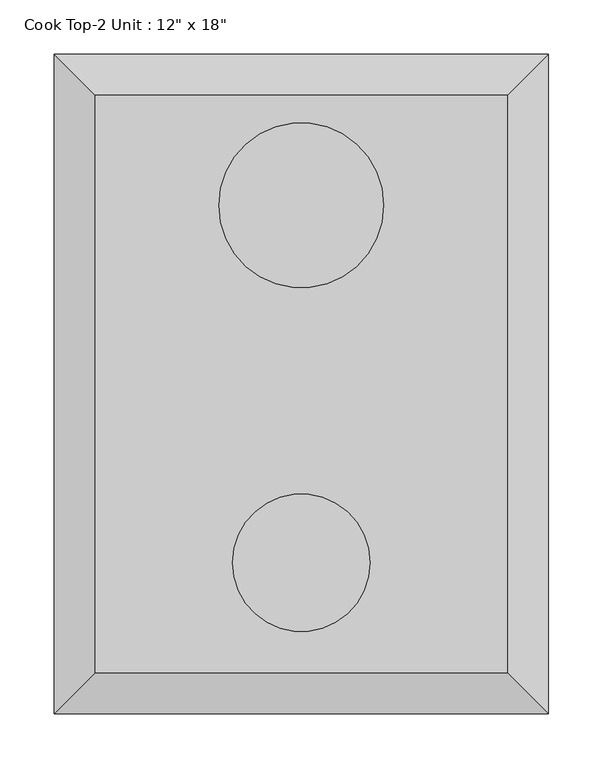
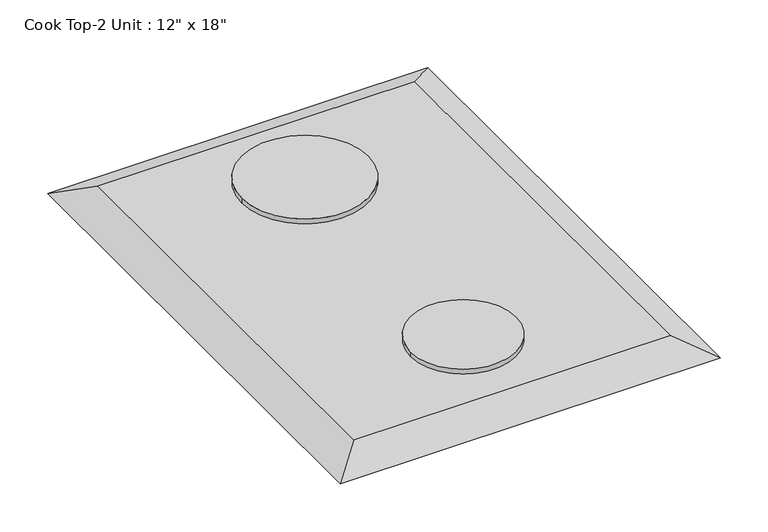
"""IFC4 building model written with IfcOpenShell, lengths in millimetres: proxy geometry."""

from ifc_helpers import new_model, si_unit, point, frame, frame_2d, origin, place, context, project, spatial, circle_curve, trimmed, segment, composite_curve, outline, extrude, faceted_brep, source, transform, mapped, element, save


def proxy_3c1fa1d0(model_context):
    return source(origin(), model_context, "Body", "SolidModel", [
        faceted_brep([(266.7, 296.9247956, 933.45), (-114.3, 296.9247956, 933.45), (-114.3, -236.4752044, 933.45), (266.7, -236.4752044, 933.45), (304.8, 335.0247956, 914.4), (304.8, -274.5752044, 914.4), (-152.4, -274.5752044, 914.4), (-152.4, 335.0247956, 914.4)], [[[0, 1, 2, 3]], [[4, 5, 6, 7]], [[4, 7, 1, 0]], [[7, 6, 2, 1]], [[6, 5, 3, 2]], [[5, 4, 0, 3]]]),
        extrude(outline(composite_curve([segment(trimmed(circle_curve(frame_2d((76.2, 195.3247956)), 76.2), [point((152.4, 195.3247956))], [point((0.0, 195.3247956))], False, "CARTESIAN"), True, "CONTINUOUS"), segment(trimmed(circle_curve(frame_2d((76.2, 195.3247956)), 76.2), [point((0.0, 195.3247956))], [point((152.4, 195.3247956))], False, "CARTESIAN"), True, "CONTINUOUS")], self_intersect=False)), frame((0.0, 0.0, 933.45), z_axis=(0.0, 0.0, 1.0), x_axis=(1.0, 0.0, 0.0)), (0.0, 0.0, 1.0), 6.35),
        extrude(outline(composite_curve([segment(trimmed(circle_curve(frame_2d((76.2, -134.8752044)), 63.5), [point((139.7, -134.8752044))], [point((12.7, -134.8752044))], False, "CARTESIAN"), True, "CONTINUOUS"), segment(trimmed(circle_curve(frame_2d((76.2, -134.8752044)), 63.5), [point((12.7, -134.8752044))], [point((139.7, -134.8752044))], False, "CARTESIAN"), True, "CONTINUOUS")], self_intersect=False)), frame((0.0, 0.0, 933.45), z_axis=(0.0, 0.0, 1.0), x_axis=(1.0, 0.0, 0.0)), (0.0, 0.0, 1.0), 6.35),
    ])


if __name__ == "__main__":
    model = new_model("IFC4")
    model_context = context("Model", 3, world=origin())
    ifc_project = project(units=[si_unit("LENGTHUNIT", "METRE", prefix="MILLI")], contexts=[model_context])
    site = spatial("IfcSite", under=ifc_project)
    building = spatial("IfcBuilding", under=site)
    placement = place(None, origin())
    proxy_shape = proxy_3c1fa1d0(model_context)
    element("IfcBuildingElementProxy", 1, Name="Cook Top-2 Unit : 12\" x 18\"", ObjectType="Cook Top-2 Unit : 12\" x 18\"", at=placement, inside=building, context=model_context, shape_type="MappedRepresentation", body=[
        mapped(proxy_shape, transform((0.0, 0.0, 0.0), x_axis=(1.0, 0.0, 0.0), y_axis=(0.0, 1.0, 0.0), z_axis=(0.0, 0.0, 1.0))),
    ])
    save(model, "model.ifc")

# Revit data of these elements
# Type "Cook Top-2 Unit : 12\" x 18\""
#   Assembly Code = "E1090400"
#   Counter Height = 3' - 0"
#   Depth = 2' - 0"
#   Width = 1' - 6"
#   Burner Material = Metal - Chrome
#   Cooktop Material = Metal - Steel, Polished
#   Default Elevation = 0
# Element 1 (IfcBuildingElementProxy, "Cook Top-2 Unit : 12\" x 18\"")
#   Materials on its faces: "Metal - Steel, Polished", "Metal - Chrome"
# Materials
#   "Metal - Chrome": colour RGB 57 57 57, transparency 0
#   "Metal - Steel, Polished": colour RGB 57 57 57, transparency 0
